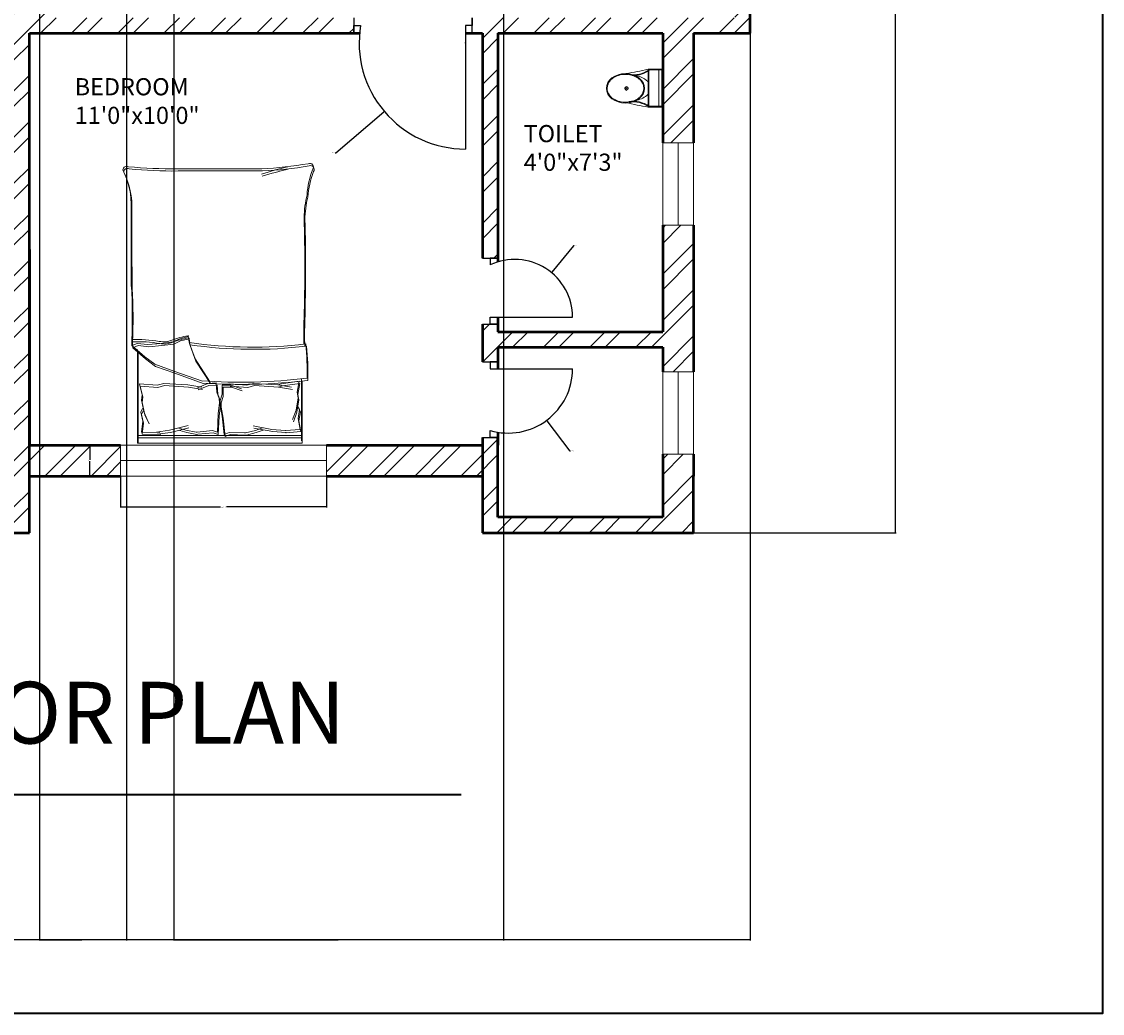
# Model space of a CAD drawing. Units: inches. Extents: x 1896 to 2572, y 1528 to 2474.
# Tile 4 of 10: x 2257 to 2572, y 1528 to 1817. Entities that reach past the tile are written whole.
import ezdxf

# ---------------------------------------------------------------- set-up
doc = ezdxf.new("R2010")
doc.units = ezdxf.units.IN
for name, color, linetype, lineweight in [('A-ANNO-DIMS', 2, 'Continuous', 18), ('A-ANNO-TTLB', 7, 'Continuous', 35), ('A-AREA-IDEN', 7, 'Continuous', 18), ('A-DOOR', 11, 'Continuous', 25), ('A-FLOR-FIXT', 8, 'Continuous', 18), ('A-FURN', 8, 'Continuous', 18), ('A-GLAZ', 131, 'Continuous', 20), ('A-WALL', 7, 'Continuous', 50)]:
    doc.layers.add(name, color=color, linetype=linetype, lineweight=lineweight)
doc.layers.add('A-WALL-PATT', color=215, linetype='Continuous', lineweight=13, true_color=0xa953a0)
doc.styles.get("Standard").update_dxf_attribs({"font": 'arial.ttf'})
doc.dimstyles.get("Standard").update_dxf_attribs({"dimtxt": 0.18, "dimasz": 0.18, "dimexe": 0.18, "dimexo": 0.0625, "dimgap": 0.09, "dimtad": 0, "dimtih": 1, "dimtoh": 1, "dimdec": 4, "dimzin": 0, "dimdsep": 46, "dimtxsty": 'Standard', "dimcen": 0.09, "dimadec": 0, "dimazin": 0, "dimtfac": 1, "dimtdec": 4, "dimtofl": 0, "dimtmove": 0, "dimatfit": 3, "dimfxl": 1, "dimtolj": 1, "dimtzin": 0, "dimarcsym": 0})

# ---------------------------------------------------------------- blocks, each defined once
blk = doc.blocks.new('A$C31115884')
for p, q in [((283, 498), (223, 498)), ((258, 466), (258, 523)), ((0, 200), (0, 0)), ((520, 200), (0, 200)), ((10, 190), (10, 10)), ((510, 190), (10, 190)), ((510, 10), (510, 190)), ((520, 0), (520, 200)), ((510, 54), (0, 54)), ((10, 10), (510, 10)), ((0, 0), (520, 0))]:
    blk.add_line(p, q)
blk.add_circle((256, 496), 23.6)
for centre, radius, start, end in [((2778, -205), 2807, 165.4549, 171.7133), ((-295, 403), 365, 324.2091, 9.3499), ((-295, 403), 375, 324.2091, 9.3499), ((806, 403), 365, 170.6501, 215.7909), ((3237, 905), 2807, 188.2867, 194.5451), ((384, 406), 293, 190.2774, 224.1564), ((139, 406), 293, 315.8436, 2.6563), ((806, 403), 375, 179.2036, 215.7909)]:
    blk.add_arc(centre, radius, start, end)
blk.add_ellipse((256, 510), major_axis=(0, -261), ratio=0.772727)
blk.add_open_spline([(256, 259), (263, 259), (270, 260), (288, 262), (299, 265), (320, 273), (330, 278), (350, 291), (360, 299), (378, 316), (386, 326), (402, 347), (409, 358), (421, 383), (427, 395), (436, 422), (440, 436), (445, 465), (447, 480), (448, 509), (448, 524), (445, 553), (443, 568), (436, 596), (432, 610), (422, 636), (416, 649), (402, 672), (395, 683), (379, 703), (370, 712), (351, 728), (341, 735), (321, 746), (310, 751), (289, 757), (278, 759), (256, 761), (245, 761), (223, 757), (212, 754), (191, 746), (181, 741), (161, 728), (151, 720), (133, 703), (125, 693), (110, 672), (103, 660), (90, 636), (85, 623), (76, 596), (72, 582), (67, 553), (66, 538), (64, 509), (65, 494), (68, 465), (70, 450), (77, 422), (81, 408), (91, 382), (97, 370), (111, 346), (118, 335), (135, 316), (144, 307), (162, 291), (172, 284), (193, 273), (203, 269), (225, 262), (236, 260), (250, 259), (253, 259), (256, 259)], degree=3, knots=[0, 0, 0, 0, 0.110105, 0.110105, 0.285049, 0.285049, 0.459994, 0.459994, 0.634938, 0.634938, 0.809882, 0.809882, 0.984827, 0.984827, 1.159771, 1.159771, 1.334715, 1.334715, 1.50966, 1.50966, 1.684604, 1.684604, 1.859549, 1.859549, 2.034493, 2.034493, 2.209437, 2.209437, 2.384382, 2.384382, 2.559326, 2.559326, 2.73427, 2.73427, 2.909215, 2.909215, 3.084159, 3.084159, 3.259103, 3.259103, 3.434048, 3.434048, 3.608992, 3.608992, 3.783936, 3.783936, 3.958881, 3.958881, 4.133825, 4.133825, 4.30877, 4.30877, 4.483714, 4.483714, 4.658658, 4.658658, 4.833603, 4.833603, 5.008547, 5.008547, 5.183491, 5.183491, 5.358436, 5.358436, 5.53338, 5.53338, 5.708324, 5.708324, 5.883269, 5.883269, 6.058213, 6.058213, 6.233158, 6.233158, 6.283185, 6.283185, 6.283185, 6.283185])
blk = doc.blocks.new('BED-DOUBLE')
for p, q in [((3.47, 63.33), (3.47, 81.44)), ((3.47, 63.33), (3.47, 81.44)), ((3.47, 81.44), (51.49, 81.44)), ((3.47, 79.91), (51.27, 79.91)), ((3.47, 79.91), (51.26, 79.91)), ((3.7, 62.69), (3.7, 80.8)), ((3.7, 62.69), (3.7, 80.8)), ((3.7, 79.27), (51.49, 79.27)), ((3.7, 79.27), (51.49, 79.27)), ((16.88, 78.42), (19.77, 79.14)), ((16.88, 78.42), (19.77, 79.14)), ((19.77, 79.14), (20.09, 79.14)), ((19.77, 79.14), (20.09, 79.14)), ((20.09, 79.14), (24.54, 78.99)), ((20.09, 79.14), (24.54, 78.99)), ((24.54, 78.99), (25.98, 79.57)), ((24.54, 78.99), (25.98, 79.57)), ((24.76, 78.36), (26.21, 78.93)), ((24.77, 78.36), (26.21, 78.93)), ((25.98, 79.57), (26.56, 74.22)), ((25.98, 79.57), (26.56, 74.22)), ((26.21, 78.93), (26.79, 73.58)), ((26.21, 78.93), (26.79, 73.58)), ((27.98, 78.95), (27.73, 73.58)), ((27.98, 78.95), (27.73, 73.58)), ((29.46, 78.46), (27.98, 78.95)), ((29.46, 78.46), (27.98, 78.95)), ((33.88, 78.89), (29.46, 78.46)), ((33.88, 78.89), (29.46, 78.46)), ((34.2, 78.91), (33.88, 78.89)), ((34.2, 78.91), (33.88, 78.89)), ((37.14, 78.37), (34.2, 78.91)), ((37.13, 78.37), (34.2, 78.91)), ((45.71, 78.9), (41.91, 78.37)), ((45.71, 78.9), (41.91, 78.37)), ((50.11, 78.89), (44.71, 78.98)), ((44.71, 78.98), (45.71, 78.9)), ((50.11, 78.89), (44.71, 78.98)), ((44.71, 78.98), (45.71, 78.9)), ((50.11, 78.89), (49.73, 75.68)), ((50.11, 78.89), (49.73, 75.68)), ((51.26, 81.44), (51.26, 54.83)), ((51.27, 81.44), (51.27, 54.83)), ((51.49, 81.44), (51.49, 80.8)), ((51.49, 80.8), (51.49, 54.19)), ((51.49, 80.8), (51.49, 54.19)), ((3.89, 78.13), (4.47, 74.95)), ((3.89, 78.13), (4.47, 74.95)), ((3.9, 78.11), (8.18, 78.43)), ((3.9, 78.11), (8.18, 78.43)), ((4.12, 77.49), (4.7, 74.31)), ((4.12, 77.49), (4.7, 74.31)), ((4.13, 77.47), (8.41, 77.8)), ((4.13, 77.47), (8.41, 77.8)), ((8.18, 78.43), (8.28, 78.42)), ((8.18, 78.43), (8.28, 78.42)), ((8.28, 78.42), (12.11, 78.13)), ((8.28, 78.42), (12.11, 78.13)), ((8.41, 77.8), (8.51, 77.78)), ((8.41, 77.8), (8.51, 77.78)), ((8.51, 77.78), (12.34, 77.49)), ((8.51, 77.78), (12.34, 77.49)), ((12.11, 78.13), (17.6, 77.12)), ((12.11, 78.13), (17.6, 77.12)), ((12.34, 77.49), (17.83, 76.48)), ((12.34, 77.49), (17.83, 76.48)), ((14.85, 77.69), (16.88, 78.42)), ((14.85, 77.69), (16.88, 78.42)), ((15.08, 77.05), (17.11, 77.78)), ((15.08, 77.05), (17.11, 77.78)), ((17.11, 77.78), (20, 78.5)), ((17.11, 77.78), (20, 78.5)), ((20, 78.5), (20.32, 78.5)), ((20, 78.5), (20.32, 78.5)), ((20.32, 78.5), (24.77, 78.36)), ((20.32, 78.5), (24.76, 78.36)), ((28.21, 78.31), (27.96, 72.94)), ((28.2, 78.31), (27.96, 72.94)), ((29.68, 77.83), (28.2, 78.31)), ((29.68, 77.83), (28.21, 78.31)), ((34.11, 78.25), (29.68, 77.83)), ((34.11, 78.25), (29.68, 77.83)), ((34.43, 78.27), (34.11, 78.25)), ((34.43, 78.27), (34.11, 78.25)), ((37.36, 77.73), (34.43, 78.27)), ((37.36, 77.73), (34.43, 78.27)), ((41.91, 78.37), (36.49, 77.02)), ((41.91, 78.37), (36.49, 77.02)), ((42.14, 77.73), (36.72, 76.38)), ((42.14, 77.73), (36.72, 76.38)), ((39.2, 77.77), (37.13, 78.37)), ((39.2, 77.77), (37.14, 78.37)), ((39.43, 77.13), (37.36, 77.73)), ((39.43, 77.13), (37.36, 77.73)), ((45.94, 78.26), (42.14, 77.73)), ((45.94, 78.26), (42.14, 77.73)), ((50.34, 78.25), (44.94, 78.34)), ((44.94, 78.34), (45.94, 78.26)), ((50.34, 78.25), (44.94, 78.34)), ((44.94, 78.34), (45.94, 78.26)), ((49.31, 73.19), (48.13, 75.87)), ((49.31, 73.19), (48.13, 75.87)), ((49.73, 75.68), (50.33, 73.11)), ((49.73, 75.68), (50.33, 73.11)), ((50.34, 78.25), (49.96, 75.04)), ((50.34, 78.25), (49.96, 75.04)), ((4.47, 74.95), (4.04, 72.34)), ((4.47, 74.95), (4.04, 72.34)), ((4.7, 74.31), (4.27, 71.7)), ((4.7, 74.31), (4.27, 71.7)), ((4.47, 68.87), (5.05, 72.49)), ((4.47, 68.87), (5.05, 72.49)), ((5.05, 72.49), (6.06, 75.24)), ((5.05, 72.49), (6.06, 75.24)), ((5.28, 71.85), (6.29, 74.6)), ((5.28, 71.85), (6.29, 74.6)), ((26.56, 74.22), (27.14, 71.04)), ((26.56, 74.22), (27.14, 71.04)), ((26.79, 73.58), (27.37, 70.4)), ((26.79, 73.58), (27.37, 70.4)), ((27.73, 73.58), (27.35, 70.37)), ((27.73, 73.58), (27.35, 70.37)), ((27.96, 72.94), (27.58, 69.73)), ((27.96, 72.94), (27.58, 69.73)), ((49.54, 72.55), (48.36, 75.23)), ((49.54, 72.55), (48.36, 75.23)), ((50.11, 69.61), (49.31, 73.19)), ((50.11, 69.61), (49.31, 73.19)), ((50.34, 68.98), (49.54, 72.55)), ((50.34, 68.98), (49.54, 72.55)), ((50.33, 73.11), (49.81, 72.06)), ((50.33, 73.11), (49.81, 72.06)), ((49.96, 75.04), (50.56, 72.47)), ((49.96, 75.04), (50.56, 72.47)), ((50.56, 72.47), (50.04, 71.42)), ((50.56, 72.47), (50.04, 71.42)), ((4.04, 72.34), (4.62, 71.33)), ((4.04, 72.34), (4.62, 71.33)), ((4.27, 71.7), (4.85, 70.69)), ((4.27, 71.7), (4.85, 70.69)), ((4.7, 68.23), (5.28, 71.85)), ((4.7, 68.23), (5.28, 71.85)), ((27.14, 69.74), (26.56, 67.86)), ((27.14, 69.74), (26.56, 67.86)), ((27.14, 71.04), (27.14, 69.74)), ((27.14, 71.04), (27.14, 69.74)), ((27.35, 70.37), (27.44, 69.07)), ((27.35, 70.37), (27.44, 69.07)), ((27.37, 70.4), (27.37, 69.1)), ((27.37, 70.4), (27.37, 69.1)), ((27.58, 69.73), (27.66, 68.43)), ((27.58, 69.73), (27.66, 68.43)), ((49.92, 68.01), (50.11, 69.61)), ((49.92, 68.01), (50.11, 69.61)), ((4.18, 64.1), (4.76, 67.28)), ((4.18, 64.1), (4.76, 67.28)), ((4.41, 63.46), (4.99, 66.64)), ((4.41, 63.46), (4.99, 66.64)), ((4.76, 67.28), (4.47, 68.87)), ((4.76, 67.28), (4.47, 68.87)), ((4.99, 66.64), (4.7, 68.23)), ((4.99, 66.64), (4.7, 68.23)), ((24.1, 65.18), (20.96, 66.27)), ((24.1, 65.18), (20.96, 66.27)), ((26.56, 67.86), (26.56, 65.18)), ((26.56, 67.86), (26.56, 65.18)), ((27.37, 69.1), (26.79, 67.22)), ((27.37, 69.1), (26.79, 67.22)), ((26.79, 67.22), (26.79, 64.54)), ((26.79, 67.22), (26.79, 64.54)), ((27.44, 69.07), (28.13, 67.23)), ((27.44, 69.07), (28.13, 67.23)), ((27.66, 68.43), (28.36, 66.59)), ((27.66, 68.43), (28.36, 66.59)), ((28.13, 67.23), (28.3, 64.55)), ((28.13, 67.23), (28.3, 64.55)), ((28.36, 66.59), (28.53, 63.91)), ((28.36, 66.59), (28.53, 63.91)), ((50.7, 64.87), (49.92, 68.01)), ((50.7, 64.87), (49.92, 68.01)), ((50.15, 67.37), (50.34, 68.98)), ((50.15, 67.37), (50.34, 68.98)), ((50.93, 64.23), (50.15, 67.37)), ((50.93, 64.23), (50.15, 67.37)), ((9.28, 64.83), (4.18, 64.1)), ((9.28, 64.83), (4.18, 64.1)), ((9.51, 64.19), (4.41, 63.46)), ((9.51, 64.19), (4.41, 63.46)), ((6.38, 65.81), (10.41, 65.15)), ((6.38, 65.81), (10.41, 65.15)), ((6.61, 65.18), (10.64, 64.51)), ((6.61, 65.18), (10.64, 64.51)), ((10.41, 65.15), (9.28, 64.83)), ((10.41, 65.15), (9.28, 64.83)), ((10.64, 64.51), (9.51, 64.19)), ((10.64, 64.51), (9.51, 64.19)), ((10.41, 65.15), (17.42, 64.72)), ((10.41, 65.15), (17.42, 64.72)), ((10.64, 64.51), (17.65, 64.08)), ((10.64, 64.51), (17.65, 64.08)), ((17.42, 64.72), (19.38, 65.27)), ((17.42, 64.72), (19.38, 65.27)), ((17.65, 64.08), (19.61, 64.63)), ((17.65, 64.08), (19.61, 64.63)), ((19.38, 65.27), (24.52, 64.87)), ((19.38, 65.27), (24.52, 64.87)), ((19.61, 64.63), (24.74, 64.23)), ((19.61, 64.63), (24.74, 64.23)), ((24.33, 64.54), (21.19, 65.63)), ((24.33, 64.54), (21.19, 65.63)), ((26.56, 65.18), (24.1, 65.18)), ((26.56, 65.18), (24.1, 65.18)), ((26.79, 64.54), (24.33, 64.54)), ((26.79, 64.54), (24.33, 64.54)), ((28.3, 64.55), (30.75, 64.7)), ((28.3, 64.55), (30.75, 64.7)), ((28.53, 63.91), (30.98, 64.06)), ((28.53, 63.91), (30.98, 64.06)), ((30.26, 64.06), (34.45, 57.57)), ((30.26, 64.06), (34.45, 57.57)), ((30.49, 63.42), (34.68, 56.93)), ((30.49, 63.42), (34.68, 56.93)), ((30.75, 64.7), (33.82, 65.99)), ((30.75, 64.7), (33.82, 65.99)), ((30.98, 64.06), (34.05, 65.35)), ((30.98, 64.06), (34.05, 65.35)), ((40.64, 61.13), (32.31, 64.06)), ((40.64, 61.13), (32.31, 64.06)), ((40.87, 60.49), (32.53, 63.42)), ((40.87, 60.49), (32.53, 63.42)), ((32.56, 65.81), (36.6, 65.15)), ((32.56, 65.81), (36.6, 65.15)), ((32.79, 65.18), (36.82, 64.51)), ((32.79, 65.18), (36.82, 64.51)), ((36.6, 65.15), (43.61, 64.72)), ((36.6, 65.15), (43.61, 64.72)), ((36.82, 64.51), (43.83, 64.08)), ((36.82, 64.51), (43.83, 64.08)), ((43.61, 64.72), (45.57, 65.27)), ((43.61, 64.72), (45.57, 65.27)), ((43.83, 64.08), (45.79, 64.63)), ((43.83, 64.08), (45.79, 64.63)), ((45.57, 65.27), (50.7, 64.87)), ((45.57, 65.27), (50.7, 64.87)), ((45.79, 64.63), (50.93, 64.23)), ((45.79, 64.63), (50.93, 64.23)), ((46.22, 59.11), (40.64, 61.13)), ((46.22, 59.11), (40.64, 61.13)), ((46.45, 58.48), (40.87, 60.49)), ((46.45, 58.48), (40.87, 60.49)), ((34.45, 57.57), (36.15, 53.08)), ((34.45, 57.57), (36.15, 53.08)), ((34.68, 56.93), (36.38, 52.44)), ((34.68, 56.93), (36.38, 52.44)), ((49.16, 56.95), (46.22, 59.11)), ((49.16, 56.95), (46.22, 59.11)), ((49.39, 56.31), (46.45, 58.48)), ((49.39, 56.31), (46.45, 58.48)), ((52.87, 53.7), (49.16, 56.95)), ((52.87, 53.7), (49.16, 56.95)), ((53.1, 53.06), (49.39, 56.31)), ((53.1, 53.06), (49.39, 56.31)), ((51.33, 53.08), (52.87, 53.7)), ((51.33, 53.08), (52.87, 53.7)), ((52.95, 51.95), (52.87, 53.7, 3.87)), ((52.95, 51.95), (52.87, 53.7, 3.87)), ((36.15, 53.08), (36.46, 51.07)), ((36.15, 53.08), (36.46, 51.07)), ((36.38, 52.44), (36.69, 50.43)), ((36.38, 52.44), (36.69, 50.43)), ((36.46, 51.07), (38.94, 51.69)), ((36.46, 51.07), (38.94, 51.69)), ((36.69, 50.43), (39.17, 51.05)), ((36.69, 50.43), (39.17, 51.05)), ((38.94, 51.69), (40.95, 52.61)), ((38.94, 51.69), (40.95, 52.61)), ((39.17, 51.05), (41.18, 51.97)), ((39.17, 51.05), (41.18, 51.97)), ((40.95, 52.61), (44.36, 53.08)), ((40.95, 52.61), (44.36, 53.08)), ((41.18, 51.97), (44.59, 52.44)), ((41.18, 51.97), (44.59, 52.44)), ((44.36, 53.08), (48.23, 53.39)), ((44.36, 53.08), (48.23, 53.39)), ((44.59, 52.44), (48.46, 52.75)), ((44.59, 52.44), (48.46, 52.75)), ((48.23, 53.39), (51.33, 53.08)), ((48.23, 53.39), (51.33, 53.08)), ((48.46, 52.75), (51.56, 52.44)), ((48.46, 52.75), (51.56, 52.44)), ((51.56, 52.44), (53.1, 53.06)), ((51.56, 52.44), (53.1, 53.06)), ((53.18, 51.31), (53.1, 53.06, 3.87)), ((53.17, 51.31), (53.1, 53.06, 3.87)), ((15.06, 2.2), (39.68, 2.2)), ((15.06, 2.2), (39.68, 2.2)), ((15.29, 1.56), (39.91, 1.56)), ((15.29, 1.56), (39.91, 1.56))]:
    blk.add_line(p, q)
for centre, radius, start, end in [((85.16, 61.35), 83.31, 178.7218, 185.604), ((85.16, 61.35), 83.31, 178.7218, 185.604), ((21.36, -100.61), 164.97, 86.0865, 96.7821), ((21.36, -100.61), 164.97, 86.0865, 96.7821), ((21.59, -101.25), 164.97, 86.0865, 96.7821), ((21.59, -101.25), 164.97, 86.0865, 96.7821), ((85.39, 60.71), 83.31, 178.7218, 185.604), ((85.39, 60.71), 83.31, 178.7218, 185.604), ((17.76, -74.87), 129.02, 81.7845, 96.9006), ((17.76, -74.87), 129.02, 81.7845, 96.9006), ((17.98, -75.51), 129.02, 81.7845, 96.9006), ((17.98, -75.51), 129.02, 81.7845, 96.9006), ((-167.31, 50.27), 170.11, 358.4762, 1.0082), ((-167.31, 50.27), 170.11, 358.4762, 1.0082), ((-167.08, 49.63), 170.11, 358.4762, 1.0082), ((-167.08, 49.63), 170.11, 358.4762, 1.0082), ((36.64, 51), 0.185, 160.2464, 271.1377), ((36.64, 51), 0.185, 160.2464, 271.1377), ((31.15, 79.96), 29.65, 280.6617, 289.8806), ((31.15, 79.96), 29.65, 280.6617, 289.8806), ((36.86, 50.36), 0.185, 160.2464, 271.1377), ((36.86, 50.36), 0.185, 160.2464, 271.1377), ((31.38, 79.32), 29.65, 280.6617, 289.8806), ((31.38, 79.32), 29.65, 280.6617, 289.8806), ((43.74, 46.38), 6.22, 78.6608, 113.7384), ((43.74, 46.38), 6.22, 78.6608, 113.7384), ((43.97, 45.74), 6.22, 78.6608, 113.7384), ((43.97, 45.74), 6.22, 78.6608, 113.7384), ((51.33, 88.1), 36.18, 259.8763, 272.5657), ((51.33, 88.1), 36.18, 259.8763, 272.5657), ((51.56, 87.46), 36.18, 259.8763, 272.5657), ((51.56, 87.46), 36.18, 259.8763, 272.5657), ((182.27, 45.13), 129.5, 176.9791, 183.8365), ((182.27, 45.13), 129.5, 176.9791, 183.8365), ((182.49, 44.49), 129.5, 176.9791, 183.8365), ((182.49, 44.49), 129.5, 176.9791, 183.8365), ((484.82, 30.83), 482.31, 178.2277, 181.7185), ((484.82, 30.83), 482.31, 178.2277, 181.7185), ((485.05, 30.19), 482.31, 178.2277, 181.7185), ((485.05, 30.19), 482.31, 178.2277, 181.7185), ((-4508.74, 13.62), 4561.86, 0.00217, 0.28689), ((-4508.74, 13.62), 4561.86, 0.00217, 0.28689), ((-4508.52, 12.98), 4561.86, 0.00217, 0.28689), ((-4508.52, 12.98), 4561.86, 0.00217, 0.28689), ((-26.9, 16.93), 29.63, 346.0648, 358.9113), ((-26.9, 16.93), 29.63, 346.0648, 358.9113), ((-26.67, 16.29), 29.63, 346.0648, 358.9113), ((-26.67, 16.29), 29.63, 346.0648, 358.9113), ((76.16, 12.78), 23.07, 177.4714, 206.4681), ((76.16, 12.78), 23.07, 177.4714, 206.4681), ((76.39, 12.14), 23.07, 177.4714, 206.4681), ((76.39, 12.14), 23.07, 177.4714, 206.4681), ((-21.66, 11.17), 23.56, 337.9751, 356.652), ((-21.66, 11.17), 23.56, 337.9751, 356.652), ((-21.43, 10.53), 23.56, 337.9751, 356.652), ((-21.43, 10.53), 23.56, 337.9751, 356.652), ((-17.22, 105.16), 106.46, 283.3832, 287.7053), ((-17.22, 105.16), 106.46, 283.3832, 287.7053), ((1.09, 1.73), 1.09, 146.1736, 293.4781), ((1.09, 1.73), 1.09, 146.1736, 293.4781), ((1.32, 1.09), 1.09, 146.1736, 293.4781), ((1.32, 1.09), 1.09, 146.1736, 293.4781), ((21.43, -119.39), 121.76, 92.9958, 99.4091), ((21.43, -119.39), 121.76, 92.9958, 99.4091), ((21.65, -120.03), 121.76, 92.9958, 99.4091), ((21.65, -120.03), 121.76, 92.9958, 99.4091), ((-16.99, 104.52), 106.46, 283.3832, 287.7053), ((-16.99, 104.52), 106.46, 283.3832, 287.7053), ((41.15, -130.83), 133.04, 84.4998, 90.6351), ((41.15, -130.83), 133.04, 84.4998, 90.6351), ((41.38, -131.47), 133.04, 84.4998, 90.6351), ((41.38, -131.47), 133.04, 84.4998, 90.6351), ((54.41, 2.57), 1.1, 242.6588, 356.02), ((54.41, 2.57), 1.1, 242.6588, 356.02), ((54.64, 1.93), 1.1, 242.6588, 356.02), ((54.64, 1.93), 1.1, 242.6588, 356.02)]:
    blk.add_arc(centre, radius, start, end)
blk = doc.blocks.new('WIN-24IN')
for p, q in [((4.5, 24), (0, 24)), ((0, 24), (9, 24)), ((0, 24), (0, 0)), ((4.5, 0), (4.5, 24)), ((9, 0), (9, 24)), ((0, 0), (9, 0)), ((9, 0), (4.5, 0))]:
    blk.add_line(p, q)
blk = doc.blocks.new('WIN-60IN')
for p, q in [((4.5, 60), (0, 60)), ((0, 60), (9, 60)), ((0, 60), (0, 0)), ((4.5, 0), (4.5, 60)), ((9, 0), (9, 60)), ((0, 0), (9, 0)), ((9, 0), (4.5, 0))]:
    blk.add_line(p, q)
blk = doc.blocks.new('*D17')
at = {"layer": 'A-ANNO-DIMS', "color": 0, "lineweight": -2, "transparency": 16777216}
for p, q in [((2285.7, 1684.34), (2285.7, 1675.22)), ((2345.7, 1684.34), (2345.7, 1675.22)), ((2285.88, 1675.4), (2314.8, 1675.4)), ((2345.52, 1675.4), (2316.59, 1675.4))]:
    blk.add_line(p, q, dxfattribs=at)
at = {"layer": 'A-ANNO-DIMS', "color": 0, "transparency": 16777216}
for points in [[(2285.88, 1675.43), (2285.88, 1675.37), (2285.7, 1675.4)], [(2345.52, 1675.43), (2345.52, 1675.37), (2345.7, 1675.4)]]:
    blk.add_solid(points, dxfattribs=at)
at = {"layer": 'Defpoints', "color": 0, "transparency": 16777216}
for p in [(2285.7, 1684.4), (2345.7, 1684.4), (2285.7, 1675.4)]:
    blk.add_point(p, dxfattribs=at)
at = {"layer": 'A-ANNO-DIMS', "color": 0, "transparency": 16777216, "insert": (2315.7, 1675.4), "char_height": 0.18, "attachment_point": 5}
blk.add_mtext('\\A1;WDW 60 TYP.', dxfattribs=at)
blk = doc.blocks.new('*D18')
at = {"layer": 'A-ANNO-DIMS', "color": 0, "lineweight": -2, "transparency": 16777216}
for p, q in [((2285.64, 1693.4), (2276.52, 1693.4)), ((2276.7, 1693.22), (2276.7, 1689.08)), ((2276.7, 1684.58), (2276.7, 1688.72)), ((2285.64, 1684.4), (2276.52, 1684.4))]:
    blk.add_line(p, q, dxfattribs=at)
at = {"layer": 'A-ANNO-DIMS', "color": 0, "transparency": 16777216}
for points in [[(2276.67, 1693.22), (2276.73, 1693.22), (2276.7, 1693.4)], [(2276.67, 1684.58), (2276.73, 1684.58), (2276.7, 1684.4)]]:
    blk.add_solid(points, dxfattribs=at)
at = {"layer": 'Defpoints', "color": 0, "transparency": 16777216}
for p in [(2276.7, 1693.4), (2285.7, 1693.4), (2285.7, 1684.4)]:
    blk.add_point(p, dxfattribs=at)
at = {"layer": 'A-ANNO-DIMS', "color": 0, "transparency": 16777216, "insert": (2276.7, 1688.9), "char_height": 0.18, "attachment_point": 5}
blk.add_mtext('\\A1;9 TYP.', dxfattribs=at)
blk = doc.blocks.new('*D19')
at = {"layer": 'A-ANNO-DIMS', "color": 0, "lineweight": -2, "transparency": 16777216}
for p, q in [((2469.12, 1813.34), (2469.12, 1549.1)), ((1962.12, 1750.34), (1962.12, 1549.1)), ((1962.3, 1549.28), (2215.33, 1549.28)), ((2468.94, 1549.28), (2215.91, 1549.28))]:
    blk.add_line(p, q, dxfattribs=at)
at = {"layer": 'A-ANNO-DIMS', "color": 0, "transparency": 16777216}
for points in [[(1962.3, 1549.31), (1962.3, 1549.25), (1962.12, 1549.28)], [(2468.94, 1549.31), (2468.94, 1549.25), (2469.12, 1549.28)]]:
    blk.add_solid(points, dxfattribs=at)
at = {"layer": 'Defpoints', "color": 0, "transparency": 16777216}
for p in [(2469.12, 1813.4), (1962.12, 1750.4), (2469.12, 1549.28)]:
    blk.add_point(p, dxfattribs=at)
at = {"layer": 'A-ANNO-DIMS', "color": 0, "transparency": 16777216, "insert": (2215.62, 1549.28), "char_height": 0.18, "attachment_point": 5}
blk.add_mtext('\\A1;507', dxfattribs=at)
blk = doc.blocks.new('*D20')
at = {"layer": 'A-ANNO-DIMS', "color": 0, "lineweight": -2, "transparency": 16777216}
for p, q in [((2180.68, 2431.4), (2511.65, 2431.4)), ((2511.47, 2431.22), (2511.47, 2049.83)), ((2511.47, 1668.08), (2511.47, 2049.47)), ((2452.68, 1667.9), (2511.65, 1667.9))]:
    blk.add_line(p, q, dxfattribs=at)
at = {"layer": 'A-ANNO-DIMS', "color": 0, "transparency": 16777216}
for points in [[(2511.44, 2431.22), (2511.5, 2431.22), (2511.47, 2431.4)], [(2511.44, 1668.08), (2511.5, 1668.08), (2511.47, 1667.9)]]:
    blk.add_solid(points, dxfattribs=at)
at = {"layer": 'Defpoints', "color": 0, "transparency": 16777216}
for p in [(2180.62, 2431.4), (2511.47, 2431.4), (2452.62, 1667.9)]:
    blk.add_point(p, dxfattribs=at)
at = {"layer": 'A-ANNO-DIMS', "color": 0, "transparency": 16777216, "insert": (2511.47, 2049.65), "char_height": 0.18, "attachment_point": 5}
blk.add_mtext('\\A1;763.5', dxfattribs=at)
blk = doc.blocks.new('*D32')
at = {"layer": 'A-ANNO-DIMS', "color": 0, "lineweight": -2, "transparency": 16777216}
for p, q in [((2301.26, 1955.84), (2301.26, 1549.1)), ((2397.26, 1955.84), (2397.26, 1549.1)), ((2301.44, 1549.28), (2349.04, 1549.28)), ((2397.08, 1549.28), (2349.48, 1549.28))]:
    blk.add_line(p, q, dxfattribs=at)
at = {"layer": 'A-ANNO-DIMS', "color": 0, "transparency": 16777216}
for points in [[(2301.44, 1549.31), (2301.44, 1549.25), (2301.26, 1549.28)], [(2397.08, 1549.31), (2397.08, 1549.25), (2397.26, 1549.28)]]:
    blk.add_solid(points, dxfattribs=at)
at = {"layer": 'Defpoints', "color": 0, "transparency": 16777216}
for p in [(2301.26, 1955.9), (2397.26, 1955.9), (2397.26, 1549.28)]:
    blk.add_point(p, dxfattribs=at)
at = {"layer": 'A-ANNO-DIMS', "color": 0, "transparency": 16777216, "insert": (2349.26, 1549.28), "char_height": 0.18, "attachment_point": 5}
blk.add_mtext('\\A1;96', dxfattribs=at)
blk = doc.blocks.new('*D35')
at = {"layer": 'A-ANNO-DIMS', "color": 0, "lineweight": -2, "transparency": 16777216}
for p, q in [((2262.12, 2373.34), (2262.12, 1549.1)), ((2287.46, 2373.34), (2287.46, 1549.1)), ((2262.3, 1549.28), (2274.4, 1549.28)), ((2287.28, 1549.28), (2275.19, 1549.28))]:
    blk.add_line(p, q, dxfattribs=at)
at = {"layer": 'A-ANNO-DIMS', "color": 0, "transparency": 16777216}
for points in [[(2262.3, 1549.31), (2262.3, 1549.25), (2262.12, 1549.28)], [(2287.28, 1549.31), (2287.28, 1549.25), (2287.46, 1549.28)]]:
    blk.add_solid(points, dxfattribs=at)
at = {"layer": 'Defpoints', "color": 0, "transparency": 16777216}
for p in [(2262.12, 2373.4), (2287.46, 2373.4), (2287.46, 1549.28)]:
    blk.add_point(p, dxfattribs=at)
at = {"layer": 'A-ANNO-DIMS', "color": 0, "transparency": 16777216, "insert": (2274.79, 1549.28), "char_height": 0.18, "attachment_point": 5}
blk.add_mtext('\\A1;25.34', dxfattribs=at)
blk = doc.blocks.new('*D37')
at = {"layer": 'A-ANNO-DIMS', "color": 0, "lineweight": -2, "transparency": 16777216}
for p, q in [((2386.04, 1810.57), (2386.22, 1810.57)), ((2386.13, 1810.48), (2386.13, 1810.66)), ((2348.38, 1778.58), (2362.4, 1790.46)), ((2348.2, 1778.58), (2348.38, 1778.58))]:
    blk.add_line(p, q, dxfattribs=at)
at = {"layer": 'A-ANNO-DIMS', "color": 0, "transparency": 16777216}
blk.add_solid([(2362.38, 1790.49), (2362.42, 1790.44), (2362.54, 1790.58)], dxfattribs=at)
at = {"layer": 'Defpoints', "color": 0, "transparency": 16777216}
for p in [(2386.13, 1810.57), (2362.54, 1790.58)]:
    blk.add_point(p, dxfattribs=at)
at = {"layer": 'A-ANNO-DIMS', "color": 0, "transparency": 16777216, "insert": (2347.72, 1778.58), "char_height": 0.18, "attachment_point": 5}
blk.add_mtext('\\A1;R30.93', dxfattribs=at)
blk = doc.blocks.new('*D48')
at = {"layer": 'A-ANNO-DIMS', "color": 0, "lineweight": -2, "transparency": 16777216}
for p, q in [((2398.53, 1715.67), (2398.71, 1715.67)), ((2398.62, 1715.58), (2398.62, 1715.76)), ((2416.62, 1691.67), (2409.98, 1700.53)), ((2416.8, 1691.67), (2416.62, 1691.67))]:
    blk.add_line(p, q, dxfattribs=at)
at = {"layer": 'A-ANNO-DIMS', "color": 0, "transparency": 16777216}
blk.add_solid([(2410, 1700.55), (2409.96, 1700.51), (2409.87, 1700.67)], dxfattribs=at)
at = {"layer": 'Defpoints', "color": 0, "transparency": 16777216}
for p in [(2398.62, 1715.67), (2409.87, 1700.67)]:
    blk.add_point(p, dxfattribs=at)
at = {"layer": 'A-ANNO-DIMS', "color": 0, "transparency": 16777216, "insert": (2417.28, 1691.67), "char_height": 0.18, "attachment_point": 5}
blk.add_mtext('\\A1;R18.75', dxfattribs=at)
blk = doc.blocks.new('*D52')
at = {"layer": 'A-ANNO-DIMS', "color": 0, "lineweight": -2, "transparency": 16777216}
for p, q in [((2417.64, 1751.46), (2411.34, 1743.8)), ((2417.82, 1751.46), (2417.64, 1751.46)), ((2400.45, 1730.66), (2400.63, 1730.66)), ((2400.54, 1730.57), (2400.54, 1730.75))]:
    blk.add_line(p, q, dxfattribs=at)
at = {"layer": 'A-ANNO-DIMS', "color": 0, "transparency": 16777216}
blk.add_solid([(2411.32, 1743.82), (2411.37, 1743.78), (2411.23, 1743.66)], dxfattribs=at)
at = {"layer": 'Defpoints', "color": 0, "transparency": 16777216}
for p in [(2411.23, 1743.66), (2400.54, 1730.66)]:
    blk.add_point(p, dxfattribs=at)
at = {"layer": 'A-ANNO-DIMS', "color": 0, "transparency": 16777216, "insert": (2418.37, 1751.46), "char_height": 0.18, "attachment_point": 5}
blk.add_mtext('\\A1;R16.834', dxfattribs=at)

msp = doc.modelspace()

# ---------------------------------------------------------------- hatches: boundary and pattern name
at = {"layer": 'A-WALL-PATT'}
h = msp.add_hatch(dxfattribs=at)
h.set_pattern_fill('ANSI32', color=256)
h.paths.add_polyline_path([(2071.6224, 2382.3979), (2071.6224, 2422.3979), (2110.6224, 2422.3979), (2110.6224, 2382.3979), (2110.6224, 2357.5961), (2119.6224, 2357.5961), (2119.6224, 2422.3979), (2171.6224, 2422.3979), (2171.6224, 2373.3979), (2193.5093, 2373.3979), (2193.5093, 2377.8979), (2193.5093, 2382.3979), (2180.6224, 2382.3979), (2180.6224, 2431.3979), (2171.6224, 2431.3979), (2119.6224, 2431.3979), (2110.6224, 2431.3979), (2062.6224, 2431.3979), (2062.6224, 2422.3979), (2062.6224, 2382.3979), (1978.6224, 2382.3979), (1978.6224, 2313.0337), (1987.6224, 2313.0337), (1987.6224, 2373.3979), (2062.6224, 2373.3979), (2067.1224, 2373.3979), (2067.1224, 2353.7982), (2071.6224, 2353.8883)])
h.paths.add_polyline_path([(2287.4624, 2382.3979), (2229.5093, 2382.3979), (2229.5093, 2373.3979), (2253.1224, 2373.3979), (2253.1224, 2175.8979), (2247.1039, 2175.8979), (2247.1039, 2166.8979), (2253.1224, 2166.8979), (2253.1224, 2150.8283), (2262.1224, 2150.8283), (2262.1224, 2166.8979), (2262.1224, 2236.8979), (2349.0731, 2236.8979), (2349.0731, 2239.1479), (2349.0731, 2241.3979), (2262.1224, 2241.3979), (2262.1224, 2373.3979), (2287.4624, 2373.3979)])
h.paths.add_polyline_path([(2452.6224, 2382.3979), (2347.4624, 2382.3979), (2347.4624, 2373.3979), (2382.1224, 2373.3979), (2382.1224, 2334.0335), (2386.6224, 2334.0335), (2386.6224, 2373.3979), (2443.6224, 2373.3979), (2443.6224, 2316.2056), (2452.6224, 2316.2056)])
h.paths.add_polyline_path([(2452.6224, 2292.2056), (2448.1224, 2292.2056), (2443.6224, 2292.2056), (2443.6224, 2292.0047), (2443.6224, 2280.9372), (2443.6224, 2268.3979), (2386.6224, 2268.3979), (2386.6224, 2312.4044), (2384.3724, 2312.4044), (2382.1224, 2312.4044), (2382.1224, 2241.3979), (2379.1336, 2241.3979), (2379.1336, 2236.8979), (2386.6224, 2236.8979), (2386.6224, 2263.8979), (2443.6224, 2263.8979), (2443.6224, 2248.8449), (2452.6224, 2248.8449)])
h.paths.add_polyline_path([(2364.1285, 2116.8979), (2262.1224, 2116.8979), (2262.1224, 2120.5401), (2257.6224, 2120.5401), (2253.1224, 2120.5401), (2253.1224, 2107.8979), (2262.1224, 2107.8979), (2269.354, 2107.8979), (2269.354, 2094.0702), (2278.354, 2094.0702), (2278.354, 2107.8979), (2347.6224, 2107.8979), (2347.6224, 2039.8979), (2278.354, 2039.8979), (2278.354, 2054.7605), (2269.354, 2054.7605), (2269.354, 2030.8979), (2278.354, 2030.8979), (2443.6224, 2030.8979), (2443.6224, 2015.198), (2452.6224, 2015.198), (2452.6224, 2030.8979), (2464.6224, 2030.8979), (2469.1224, 2030.8979), (2469.1224, 2117.0352), (2452.6767, 2116.9466), (2452.6285, 2125.8979), (2452.6224, 2125.8979), (2452.6224, 2212.8449), (2443.6224, 2212.8449), (2443.6224, 2116.8979), (2385.832, 2116.8979), (2385.832, 2112.3979), (2385.832, 2107.8979), (2464.6224, 2107.8979), (2464.6224, 2039.8979), (2443.6224, 2039.8979), (2356.6224, 2039.8979), (2356.6224, 2107.8979), (2364.1285, 2107.8979)])
h.paths.add_polyline_path([(2452.6224, 1967.198), (2443.6224, 1967.198), (2443.6224, 1955.8979), (2259.1224, 1955.8979), (2254.6224, 1955.8979), (2254.6224, 1941.6358), (2263.6224, 1941.6358), (2263.6224, 1946.8979), (2379.1224, 1946.8979), (2379.1224, 1913.0204), (2383.6224, 1913.0204), (2383.6224, 1946.8979), (2443.6224, 1946.8979), (2443.6224, 1930.729), (2452.6224, 1930.729)])
h.paths.add_polyline_path([(2469.1224, 1871.8979), (2464.6224, 1871.8979), (2452.6224, 1871.8979), (2452.6224, 1894.729), (2443.6224, 1894.729), (2443.6224, 1871.8979), (2388.1304, 1871.8979), (2388.1304, 1867.3979), (2443.6224, 1867.3979), (2464.6224, 1867.3979), (2464.6224, 1817.8979), (2443.6224, 1817.8979), (2388.1304, 1817.8979), (2388.1304, 1815.6479), (2388.1304, 1813.3979), (2391.1224, 1813.3979), (2391.1224, 1747.8899), (2395.6224, 1747.8899), (2395.6224, 1813.3979), (2443.6224, 1813.3979), (2443.6224, 1781.4434), (2452.6224, 1781.4434), (2452.6224, 1813.3979), (2464.6224, 1813.3979), (2469.1224, 1813.3979)])
h.paths.add_polyline_path([(2263.6224, 1910.9737), (2259.1224, 1910.9737), (2254.6224, 1910.9737), (2254.6224, 1889.8979), (2251.2778, 1889.8979), (2251.2778, 1880.8979), (2254.6224, 1880.8979), (2254.6224, 1817.8979), (2254.6224, 1754.8979), (2254.6224, 1693.3979), (2254.6224, 1684.3979), (2254.6224, 1672.3979), (2200.6224, 1672.3979), (2200.6224, 1684.3979), (2200.6224, 1693.3979), (2200.6224, 1754.8979), (2196.1224, 1754.8979), (2196.1224, 1693.3979), (2150.0488, 1693.3979), (2150.0488, 1684.3979), (2196.1224, 1684.3979), (2196.1224, 1672.3979), (2196.1224, 1667.8979), (2254.6224, 1667.8979), (2259.1224, 1667.8979), (2259.1224, 1693.3979), (2259.1224, 1813.3979), (2353.6224, 1813.3979), (2353.6224, 1815.6479), (2353.6224, 1817.8979), (2263.6224, 1817.8979)])
h.paths.add_polyline_path([(2391.1224, 1693.3979), (2345.6981, 1693.3979), (2345.6981, 1684.3979), (2391.1224, 1684.3979)])
h.paths.add_polyline_path([(2285.6981, 1693.3979), (2259.1224, 1693.3979), (2259.1224, 1684.3979), (2285.6981, 1684.3979), (2285.6981, 1688.8979)], flags=17)
h.paths.add_polyline_path([(2452.6224, 1757.4434), (2448.1224, 1757.4434), (2443.6224, 1757.4434), (2443.6224, 1726.3979), (2395.6224, 1726.3979), (2395.6224, 1728.6572), (2393.3724, 1728.6572), (2391.1224, 1728.6572), (2391.1224, 1717.6723), (2395.6224, 1717.6723), (2395.6224, 1721.8979), (2443.6224, 1721.8979), (2443.6224, 1714.8), (2452.6224, 1714.8)])
h.paths.add_polyline_path([(2452.6224, 1684.3979), (2452.6224, 1690.8), (2443.6224, 1690.8), (2443.6224, 1679.8979), (2443.6224, 1672.3979), (2395.6224, 1672.3979), (2395.6224, 1695.6708), (2391.1224, 1695.5986), (2391.1224, 1672.3979), (2391.1224, 1667.8979), (2452.6224, 1667.8979)])
h.paths.add_polyline_path([(1987.6224, 1880.8979), (2068.6224, 1880.8979), (2125.6224, 1880.8979), (2125.6224, 1788.8466), (2130.1224, 1788.8466), (2130.1224, 1880.8979), (2216.1958, 1880.8979), (2216.1958, 1885.3979), (2216.1958, 1889.8979), (2208.1224, 1889.8979), (2208.1224, 1996.3717), (2203.6224, 1996.3717), (2199.1224, 1996.3717), (2199.1224, 1889.8979), (2073.1224, 1889.8979), (2073.1224, 1917.1874), (2068.6224, 1917.1874), (2068.6224, 1889.8979), (1987.6224, 1889.8979), (1987.6224, 1912.4976), (1978.6224, 1912.4976), (1978.6224, 1805.5193), (1987.6224, 1805.5193)])
h.paths.add_polyline_path([(2019.9303, 1754.8979), (1987.6224, 1754.8979), (1966.6224, 1754.8979), (1966.6224, 1801.0193), (1987.6224, 1801.0193), (1987.6224, 1805.5193), (1962.1224, 1805.5193), (1962.1224, 1750.3979), (1966.6224, 1750.3979), (1978.6224, 1750.3979), (1987.6224, 1750.3979), (2019.9303, 1750.3979)])
h.paths.add_polyline_path([(2135.5566, 1754.8979), (2130.1224, 1754.8979), (2130.1224, 1758.052), (2127.8724, 1758.052), (2125.6224, 1758.052), (2125.6224, 1754.8979), (2068.6224, 1754.8979), (2043.2292, 1754.8979), (2043.2292, 1750.3979), (2068.6224, 1750.3979), (2098.6224, 1750.3979), (2098.6224, 1693.3979), (2068.6224, 1693.3979), (1987.6224, 1693.3979), (1987.6224, 1707.3003), (1983.1224, 1707.3003), (1978.6224, 1707.3003), (1978.6224, 1684.3979), (2068.6224, 1684.3979), (2126.0488, 1684.3979), (2126.0488, 1688.8979), (2126.0488, 1693.3979), (2103.1224, 1693.3979), (2103.1224, 1750.3979), (2130.1224, 1750.3979), (2135.5566, 1750.3979)])
h.paths.add_polyline_path([(1987.6224, 1750.3979), (1978.6224, 1750.3979), (1978.6224, 1731.3003), (1987.6224, 1731.3003)], flags=0)
h.paths.add_polyline_path([(1987.6224, 1973.8979), (2068.6224, 1973.8979), (2073.1224, 1973.8979), (2073.1224, 1978.3979), (1971.1224, 1978.3979), (1971.1224, 2030.3979), (1978.6224, 2030.3979), (1987.6224, 2030.3979), (2104.9199, 2030.3979), (2104.9199, 2032.6479), (2104.9199, 2034.8979), (1987.6224, 2034.8979), (1971.1224, 2034.8979), (1971.1224, 2085.8979), (2003.6464, 2085.8979), (2003.6464, 2090.3979), (1987.6224, 2090.3979), (1987.6224, 2166.8979), (2115.1224, 2166.8979), (2137.6224, 2166.8979), (2137.6224, 2114.4229), (2142.1224, 2114.4229), (2142.1224, 2124.8979), (2153.5306, 2124.8979), (2153.5306, 2127.1479), (2153.5306, 2129.3979), (2142.1224, 2129.3979), (2142.1224, 2166.8979), (2199.1224, 2166.8979), (2199.1224, 2129.3979), (2177.5306, 2129.3979), (2177.5306, 2124.8979), (2199.1224, 2124.8979), (2199.1224, 2034.8979), (2142.1224, 2034.8979), (2142.1224, 2091.6671), (2139.8724, 2091.6671), (2137.6224, 2091.6671), (2137.6224, 2034.8979), (2133.8326, 2034.8979), (2133.8326, 2030.3979), (2137.6224, 2030.3979), (2142.1224, 2030.3979), (2199.1224, 2030.3979), (2199.1224, 2024.2654), (2208.1224, 2024.2654), (2208.1224, 2030.3979), (2208.1224, 2166.8979), (2214.5775, 2166.8979), (2214.5775, 2171.3979), (2214.5775, 2175.8979), (2115.1224, 2175.8979), (2115.1224, 2329.9154), (2112.4137, 2329.9154), (2110.6224, 2329.9154), (2110.6224, 2175.8979), (2082.1224, 2175.8979), (2082.1224, 2202.6443), (2079.8724, 2202.6443), (2077.6224, 2202.6443), (2077.6224, 2175.8979), (1987.6224, 2175.8979), (1987.6224, 2191.3531), (1983.1224, 2191.3531), (1978.6224, 2191.3531), (1978.6224, 2090.3979), (1966.6224, 2090.3979), (1966.6224, 2085.8979), (1966.6224, 2030.3979), (1966.6224, 1973.8979), (1978.6224, 1973.8979), (1978.6224, 1948.4976), (1983.1224, 1948.4976), (1987.6224, 1948.4976)])
h.paths.add_polyline_path([(1987.6224, 2253.0337), (1983.1224, 2253.0337), (1978.6224, 2253.0337), (1978.6224, 2215.3531), (1987.6224, 2215.3531), (1987.6224, 2224.8979), (2077.6224, 2224.8979), (2077.6224, 2221.9854), (2082.1224, 2221.9854), (2082.1224, 2229.3979), (1987.6224, 2229.3979)], flags=17)
h.paths.add_polyline_path([(2220.5047, 1978.7278), (2253.7278, 1978.7278), (2253.7278, 1997.3851), (2220.5047, 1997.3851)], flags=9)
h.paths.add_polyline_path([(2303.6746, 2064.9806), (2320.5334, 2064.9806), (2320.5334, 2075.2842), (2303.6746, 2075.2842)], flags=25)

# ---------------------------------------------------------------- linework, layer by layer
at = {"layer": 'A-ANNO-TTLB'}
msp.add_line((2109.7357, 1591.6303), (2384.9301, 1591.6303), dxfattribs=at)
msp.add_lwpolyline([(1895.84, 2455.9668), (2571.702, 2455.9668), (2571.702, 1527.8833), (1895.84, 1527.8833)], close=True, dxfattribs=at)
at = {"layer": 'A-DOOR'}
for p, q in [((2353.6224, 1817.8979), (2353.6224, 1813.3979)), ((2388.1304, 1813.3979), (2388.1304, 1817.8979)), ((2388.1304, 1817.8979), (2388.1304, 1815.6479)), ((2353.6224, 1813.3979), (2353.6224, 1815.6479)), ((2353.6224, 1815.6479), (2355.6224, 1815.6479)), ((2388.1304, 1815.6479), (2386.1304, 1815.6479)), ((2386.1304, 1815.6479), (2386.1304, 1791.6479)), ((2386.1304, 1791.6479), (2386.1304, 1779.6479)), ((2391.1224, 1747.8899), (2395.6224, 1747.8899)), ((2395.6224, 1747.8899), (2393.3724, 1747.8899)), ((2393.3724, 1747.8899), (2393.3724, 1745.8899)), ((2391.1224, 1728.6572), (2395.6224, 1728.6572)), ((2393.3724, 1728.6572), (2393.3724, 1730.6572)), ((2393.3724, 1730.6572), (2417.3724, 1730.6572)), ((2395.6224, 1728.6572), (2393.3724, 1728.6572)), ((2391.1224, 1717.6723), (2395.6224, 1717.6723)), ((2395.6224, 1717.6723), (2393.3724, 1717.6723)), ((2393.3724, 1717.6723), (2393.3724, 1715.6723)), ((2393.3724, 1715.6723), (2417.3724, 1715.6723)), ((2393.3724, 1695.6708), (2393.3724, 1697.6708)), ((2391.1224, 1695.5986), (2395.6224, 1695.6708)), ((2395.6224, 1695.6708), (2393.3724, 1695.6708))]:
    msp.add_line(p, q, dxfattribs=at)
for centre, radius, start, end in [((2386.1304, 1810.5748), 30.9269, 170.558841, 270), ((2400.5384, 1730.6572), 16.834, 360, 115.19396), ((2398.6213, 1715.6723), 18.7511, 253.744322, 360)]:
    msp.add_arc(centre, radius, start, end, dxfattribs=at)
at = {"layer": 'A-WALL'}
for p, q in [((2469.1224, 1813.3979), (2469.1224, 1871.8979)), ((2259.1224, 1693.3979), (2259.1224, 1813.3979)), ((2259.1224, 1813.3979), (2355.3326, 1813.3979)), ((2386.1304, 1813.3979), (2391.1224, 1813.3979)), ((2391.1224, 1813.3979), (2391.1224, 1747.8899)), ((2395.6224, 1813.3979), (2443.6224, 1813.3979)), ((2395.6224, 1813.3979), (2395.6224, 1746.7575)), ((2443.6224, 1813.3979), (2443.6224, 1781.4434)), ((2452.6224, 1813.3979), (2464.6224, 1813.3979)), ((2452.6224, 1813.3979), (2452.6224, 1781.4434)), ((2464.6224, 1813.3979), (2469.1224, 1813.3979)), ((2443.6224, 1757.4434), (2443.6224, 1726.3979)), ((2452.6224, 1757.4434), (2452.6224, 1714.8)), ((2259.1224, 1750.3979), (2259.1224, 1754.8979)), ((2259.1224, 1750.3979), (2259.1224, 1693.3979)), ((2391.1224, 1728.6572), (2391.1224, 1717.6723)), ((2395.6224, 1730.6572), (2395.6224, 1726.3979)), ((2395.6224, 1726.3979), (2443.6224, 1726.3979)), ((2395.6224, 1721.8979), (2443.6224, 1721.8979)), ((2395.6224, 1721.8979), (2395.6224, 1715.6723)), ((2443.6224, 1721.8979), (2443.6224, 1714.8)), ((2443.6224, 1721.8979), (2443.6224, 1714.8)), ((2395.6224, 1697.1625), (2395.6224, 1693.3979)), ((2391.1224, 1695.5986), (2391.1224, 1672.3979)), ((2391.1224, 1695.5986), (2391.1224, 1693.3979)), ((2395.6224, 1672.3979), (2395.6224, 1695.6708)), ((2259.1224, 1667.8979), (2259.1224, 1693.3979)), ((2259.1224, 1693.3979), (2285.6981, 1693.3979)), ((2345.6981, 1693.3979), (2391.1224, 1693.3979)), ((2443.6224, 1690.8), (2443.6224, 1679.8979)), ((2452.6224, 1690.8), (2452.6224, 1684.3979)), ((2259.1224, 1684.3979), (2285.6981, 1684.3979)), ((2345.6981, 1684.3979), (2391.1224, 1684.3979)), ((2443.6224, 1684.3979), (2443.6224, 1672.3979)), ((2452.6224, 1667.8979), (2452.6224, 1684.3979)), ((2391.1224, 1672.3979), (2391.1224, 1667.8979)), ((2443.6224, 1672.3979), (2395.6224, 1672.3979)), ((2254.6224, 1667.8979), (2259.1224, 1667.8979)), ((2391.1224, 1667.8979), (2452.6224, 1667.8979))]:
    msp.add_line(p, q, dxfattribs=at)

# ---------------------------------------------------------------- block references
at = {"layer": 'A-FLOR-FIXT', "xscale": 0.021283599635143, "yscale": 0.021283599635143, "zscale": 0.021283599635143, "rotation": 89.99999999999999}
msp.add_blockref('A$C31115884', (2443.6224, 1791.8869), dxfattribs=at)
at = {"layer": 'A-FURN', "rotation": 180}
msp.add_blockref('BED-DOUBLE', (2342.1153, 1775.4632), dxfattribs=at)
at = {"layer": 'A-GLAZ'}
for name, p, rotation in [('WIN-24IN', (2452.6229, 1781.4435), 180), ('WIN-60IN', (2345.6978, 1684.3974), 90)]:
    msp.add_blockref(name, p, dxfattribs=dict(at, rotation=rotation))
at = {"layer": 'A-GLAZ', "extrusion": (0, 0, -1), "zscale": -1}
msp.add_blockref('WIN-24IN', (-2452.6229, 1690.8), dxfattribs=at)

# ---------------------------------------------------------------- texts
at = {"layer": 'A-ANNO-TTLB', "insert": (2133.9082, 1624.467), "char_height": 18, "attachment_point": 1}
msp.add_mtext_dynamic_manual_height_columns('FIRST FLOOR PLAN', width=466.151735, gutter_width=12.5, heights=[0], dxfattribs=at)
at = {"layer": 'A-AREA-IDEN', "char_height": 5, "attachment_point": 1}
for s, width, insert in [('BEDROOM\\P11\'0"x10\'0"', 131.359446, (2272.3412, 1800.3028)), ('TOILET\\P4\'0"x7\'3"', 114.953922, (2403.1271, 1786.6482))]:
    msp.add_mtext_dynamic_manual_height_columns(s, width=width, gutter_width=12.5, heights=[0], dxfattribs=dict(at, insert=insert))

# ---------------------------------------------------------------- dimensions: what is measured, and where the dimension line sits
at = {"layer": 'A-ANNO-DIMS'}
dim = msp.add_linear_dim(base=(2511.4724, 2431.3979), p1=(2452.6224, 1667.8979), p2=(2180.6224, 2431.3979), angle=90, dimstyle='Standard', override={"dimdec": 1, "dimlfac": 1, "dimrnd": 0, "dimzin": 0, "dimdsep": 46, "dimlunit": 2}, dxfattribs=at)
dim.commit()
dim.dimension.update_dxf_attribs({"geometry": '*D20', "text_midpoint": (2511.4724, 2049.6479)})
for base, p1, p2, override, picture, middle in [((2287.4624, 1549.2803), (2262.1224, 2373.3979), (2287.4624, 2373.3979), {"dimdec": 2, "dimlfac": 1, "dimrnd": 0, "dimzin": 0, "dimdsep": 46, "dimlunit": 2}, '*D35', (2274.7924, 1549.2803)), ((2397.2636, 1549.2803), (2301.2636, 1955.8979), (2397.2636, 1955.8979), {"dimdec": 0, "dimlfac": 1, "dimrnd": 0, "dimzin": 0, "dimdsep": 46, "dimlunit": 2}, '*D32', (2349.2636, 1549.2803)), ((2469.1224, 1549.2803), (1962.1224, 1750.3979), (2469.1224, 1813.3979), {"dimdec": 0, "dimlfac": 1, "dimrnd": 0, "dimzin": 0, "dimdsep": 46, "dimlunit": 2}, '*D19', (2215.6224, 1549.2803))]:
    dim = msp.add_linear_dim(base=base, p1=p1, p2=p2, dimstyle='Standard', override=override, dxfattribs=at)
    dim.commit()
    dim.dimension.update_dxf_attribs({"geometry": picture, "text_midpoint": middle})
for center, mpoint, override, picture, middle in [((2386.1304, 1810.5748), (2362.5362, 1790.5802), {"dimdec": 2, "dimlfac": 1, "dimrnd": 0, "dimzin": 0, "dimdsep": 46, "dimlunit": 2}, '*D37', (2347.7198, 1778.5834)), ((2400.5384, 1730.6572), (2411.2284, 1743.6614), {"dimdec": 3, "dimlfac": 1, "dimrnd": 0, "dimzin": 0, "dimdsep": 46, "dimlunit": 2}, '*D52', (2418.3718, 1751.4639)), ((2398.6213, 1715.6723), (2409.8729, 1700.6721), {"dimdec": 2, "dimlfac": 1, "dimrnd": 0, "dimzin": 0, "dimdsep": 46, "dimlunit": 2}, '*D48', (2417.2844, 1691.672))]:
    dim = msp.add_radius_dim(center=center, mpoint=mpoint, dimstyle='Standard', override=override, dxfattribs=at)
    dim.commit()
    dim.dimension.update_dxf_attribs({"geometry": picture, "text_midpoint": middle, "dimtype": 164})
for base, p1, p2, angle, text, picture, middle in [((2276.6981, 1693.3979), (2285.6981, 1684.3979), (2285.6981, 1693.3979), 90, '<> TYP.', '*D18', (2276.6981, 1688.8979)), ((2285.6981, 1675.3979), (2345.6981, 1684.3979), (2285.6981, 1684.3979), 180, 'WDW <> TYP.', '*D17', (2315.6981, 1675.3979))]:
    dim = msp.add_linear_dim(base=base, p1=p1, p2=p2, angle=angle, text=text, dimstyle='Standard', override={"dimdec": 0, "dimlfac": 1, "dimrnd": 0, "dimzin": 0, "dimdsep": 46, "dimlunit": 2}, dxfattribs=at)
    dim.commit()
    dim.dimension.update_dxf_attribs({"geometry": picture, "text_midpoint": middle})

doc.saveas('drawing.dxf')
